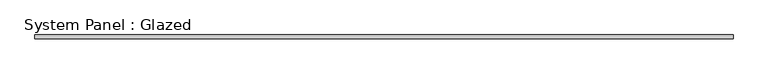
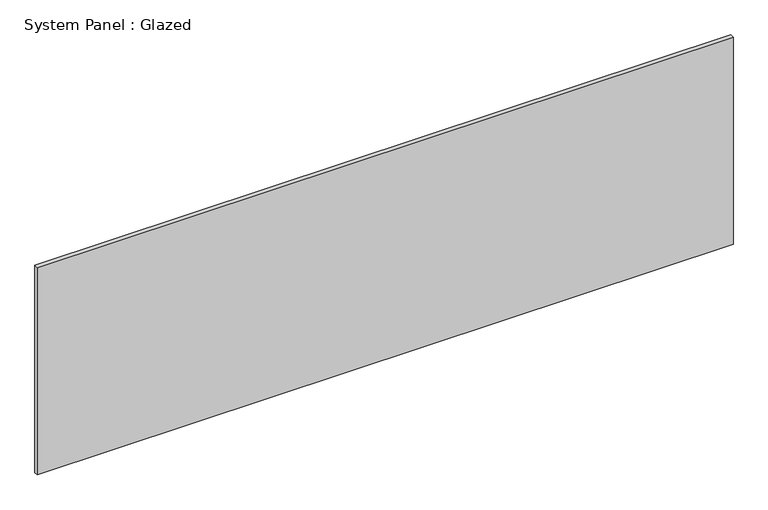
"""IFC4 building model written with IfcOpenShell, lengths in millimetres: plate geometry, System Panel : Glazed."""

from ifc_helpers import new_model, si_unit, origin, origin_with_axes, place, context, project, spatial, polyline, outline, extrude, source, transform, mapped, element, save


def system_panel_glazed_e6f20943(model_context):
    return source(origin(), model_context, "Body", "SweptSolid", [
        extrude(outline(polyline([(2320.2540045, 19.05), (-2320.2540045, 19.05), (-2320.2540045, 44.45), (2320.2540045, 44.45), (2320.2540045, 19.05)])), origin_with_axes(), (0.0, 0.0, 1.0), 1460.5),
    ])


if __name__ == "__main__":
    model = new_model("IFC4")
    model_context = context("Model", 3, world=origin())
    ifc_project = project(units=[si_unit("LENGTHUNIT", "METRE", prefix="MILLI")], contexts=[model_context])
    site = spatial("IfcSite", under=ifc_project)
    building = spatial("IfcBuilding", under=site)
    placement = place(None, origin())
    system_panel_glazed_shape = system_panel_glazed_e6f20943(model_context)
    element("IfcPlate", 1, ObjectType="System Panel : Glazed", at=placement, inside=building, context=model_context, shape_type="MappedRepresentation", body=[
        mapped(system_panel_glazed_shape, transform((0.0, 0.0, 0.0), x_axis=(1.0, 0.0, 0.0), y_axis=(0.0, 1.0, 0.0), z_axis=(0.0, 0.0, 1.0))),
    ])
    save(model, "model.ifc")

# Revit data of these elements
# Type "System Panel : Glazed"
#   Construction Type Id = "GSP4R"
#   Analytic Construction = "1/8 in Pilkington single glazing"
#   Visual Light Transmittance = 0.9
#   Solar Heat Gain Coefficient = 0.86
#   Heat Transfer Coefficient (U) = 1.18115 BTU/(h·ft²·°F)
# Element 1 (IfcPlate, "System Panel : Glazed")
#   Materials on its faces: "Glass"
# Materials
#   "Glass": class "Glass", colour RGB 0 128 192, transparency 0.75, Description = "Soda Lime Glass", Cost = 0
